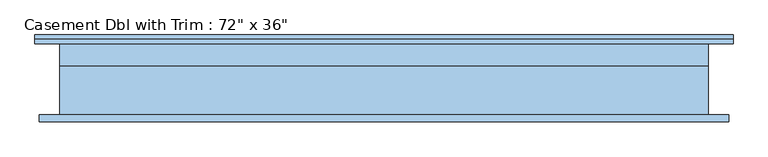
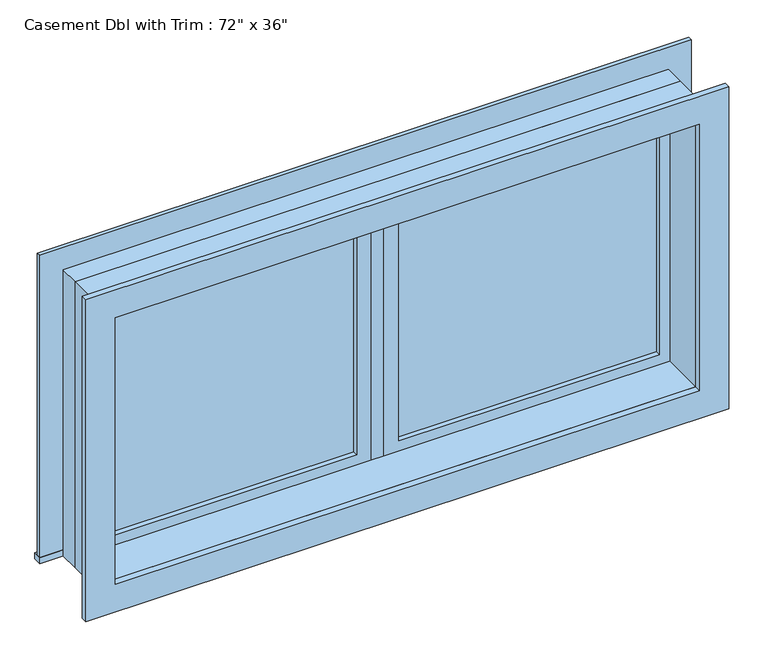
"""IFC4 building model written with IfcOpenShell, lengths in millimetres: window geometry."""

from ifc_helpers import new_model, si_unit, frame, origin, place, context, project, spatial, polyline, outline, extrude, source, transform, mapped, element, save


def window_6fce5177(model_context):
    return source(origin(), model_context, "Body", "SweptSolid", [
        extrude(outline(polyline([(63.5, 84.125), (850.9, 84.125), (850.9, 71.425), (63.5, 71.425), (63.5, 84.125)])), frame((0.0, 0.0, 1282.7), z_axis=(0.0, 0.0, 1.0), x_axis=(1.0, 0.0, 0.0)), (0.0, 0.0, 1.0), 787.4),
        extrude(outline(polyline([(2114.55, 19.05), (1238.25, 19.05), (1238.25, 895.35), (2114.55, 895.35), (2114.55, 19.05)]), holes=[polyline([(2070.1, 63.5), (2070.1, 850.9), (1282.7, 850.9), (1282.7, 63.5), (2070.1, 63.5)])]), frame((0.0, 55.55, 0.0), z_axis=(0.0, 1.0, 0.0), x_axis=(0.0, 0.0, 1.0)), (0.0, 0.0, 1.0), 44.45),
        extrude(outline(polyline([(19.05, 55.55), (-19.05, 55.55), (-19.05, 119.05), (19.05, 119.05), (19.05, 55.55)])), frame((0.0, 0.0, 1238.25), z_axis=(0.0, 0.0, 1.0), x_axis=(1.0, 0.0, 0.0)), (0.0, 0.0, 1.0), 876.3),
        extrude(outline(polyline([(-984.25, 144.45), (984.25, 144.45), (984.25, 119.05), (-984.25, 119.05), (-984.25, 144.45)])), frame((0.0, 0.0, 1219.2), z_axis=(0.0, 0.0, 1.0), x_axis=(1.0, 0.0, 0.0)), (0.0, 0.0, 1.0), 19.05),
        extrude(outline(polyline([(2114.55, -895.35), (2114.55, 895.35), (1238.25, 895.35), (1238.25, 984.25), (2203.45, 984.25), (2203.45, -984.25), (1238.25, -984.25), (1238.25, -895.35), (2114.55, -895.35)])), frame((0.0, 119.05, 0.0), z_axis=(0.0, 1.0, 0.0), x_axis=(0.0, 0.0, 1.0)), (0.0, 0.0, 1.0), 12.7),
        extrude(outline(polyline([(2190.75, 971.55), (2190.75, -971.55), (1162.05, -971.55), (1162.05, 971.55), (2190.75, 971.55)]), holes=[polyline([(2101.85, 882.65), (1250.95, 882.65), (1250.95, -882.65), (2101.85, -882.65), (2101.85, 882.65)])]), frame((0.0, -100.0, 0.0), z_axis=(0.0, 1.0, 0.0), x_axis=(0.0, 0.0, 1.0)), (0.0, 0.0, 1.0), 19.05),
        extrude(outline(polyline([(-63.5, 71.425), (-850.9, 71.425), (-850.9, 84.125), (-63.5, 84.125), (-63.5, 71.425)])), frame((0.0, 0.0, 1282.7), z_axis=(0.0, 0.0, 1.0), x_axis=(1.0, 0.0, 0.0)), (0.0, 0.0, 1.0), 787.4),
        extrude(outline(polyline([(2114.55, -895.35), (1238.25, -895.35), (1238.25, -19.05), (2114.55, -19.05), (2114.55, -895.35)]), holes=[polyline([(2070.1, -850.9), (2070.1, -63.5), (1282.7, -63.5), (1282.7, -850.9), (2070.1, -850.9)])]), frame((0.0, 55.55, 0.0), z_axis=(0.0, 1.0, 0.0), x_axis=(0.0, 0.0, 1.0)), (0.0, 0.0, 1.0), 44.45),
        extrude(outline(polyline([(2133.6, -914.4), (1219.2, -914.4), (1219.2, 914.4), (2133.6, 914.4), (2133.6, -914.4)]), holes=[polyline([(2101.85, -882.65), (2101.85, 882.65), (1250.95, 882.65), (1250.95, -882.65), (2101.85, -882.65)])]), frame((0.0, -80.95, 0.0), z_axis=(0.0, 1.0, 0.0), x_axis=(0.0, 0.0, 1.0)), (0.0, 0.0, 1.0), 136.5),
        extrude(outline(polyline([(2133.6, 914.4), (2133.6, -914.4), (1219.2, -914.4), (1219.2, 914.4), (2133.6, 914.4)]), holes=[polyline([(2114.55, 895.35), (1238.25, 895.35), (1238.25, -895.35), (2114.55, -895.35), (2114.55, 895.35)])]), frame((0.0, 55.55, 0.0), z_axis=(0.0, 1.0, 0.0), x_axis=(0.0, 0.0, 1.0)), (0.0, 0.0, 1.0), 63.5),
    ])


if __name__ == "__main__":
    model = new_model("IFC4")
    model_context = context("Model", 3, world=origin())
    ifc_project = project(units=[si_unit("LENGTHUNIT", "METRE", prefix="MILLI")], contexts=[model_context])
    site = spatial("IfcSite", under=ifc_project)
    building = spatial("IfcBuilding", under=site)
    placement = place(None, origin())
    window_shape = window_6fce5177(model_context)
    element("IfcWindow", 1, ObjectType="Casement Dbl with Trim : 72\" x 36\"", at=placement, inside=building, context=model_context, shape_type="MappedRepresentation", body=[
        mapped(window_shape, transform((0.0, 0.0, 0.0), x_axis=(1.0, 0.0, 0.0), y_axis=(0.0, 1.0, 0.0), z_axis=(0.0, 0.0, 1.0))),
    ])
    save(model, "model.ifc")

# Revit data of these elements
# Type "Casement Dbl with Trim : 72\" x 36\""
#   Type Mark = "20"
#   Construction Type Id = "GSP4R"
#   Assembly Code = "B2020100"
#   Analytic Construction = "1/8 in Pilkington single glazing"
#   Visual Light Transmittance = 0.9
#   Solar Heat Gain Coefficient = 0.78
#   Heat Transfer Coefficient (U) = 3.6886 W/(m²·K)
#   Height = 3' - 0"
#   Default Sill Height = 4' - 0"
#   Trim Projection - Ext. = 0' - 0 1/2"
#   Trim Projection - Int. = 0' - 0 3/4"
#   Trim Width - Exterior = 0' - 3 1/2"
#   Trim Width - Interior = 0' - 3 1/2"
#   Width = 6' - 0"
#   Window Inset = 0' - 0 3/4"
#   Define Thermal Properties by = 1
#   Glass Pane Material = Glass
#   Sash Material = Sash
#   Trim Exterior Material = Trim
#   Trim Interior Material = Trim
#   Wall Closure = (empty or 0)
# Element 1 (IfcWindow, "Casement Dbl with Trim : 72\" x 36\"")
#   Materials on its faces: "Sash", "Trim", "Glass"
# Materials
#   "Glass": class "Glass", colour RGB 218 227 224, transparency 0.85, Description = "Soda Lime Glass", Cost = 0
#   "Sash": class "Wood", colour RGB 136 99 55, transparency 0
#   "Trim": class "Wood", colour RGB 224 178 126, transparency 0
